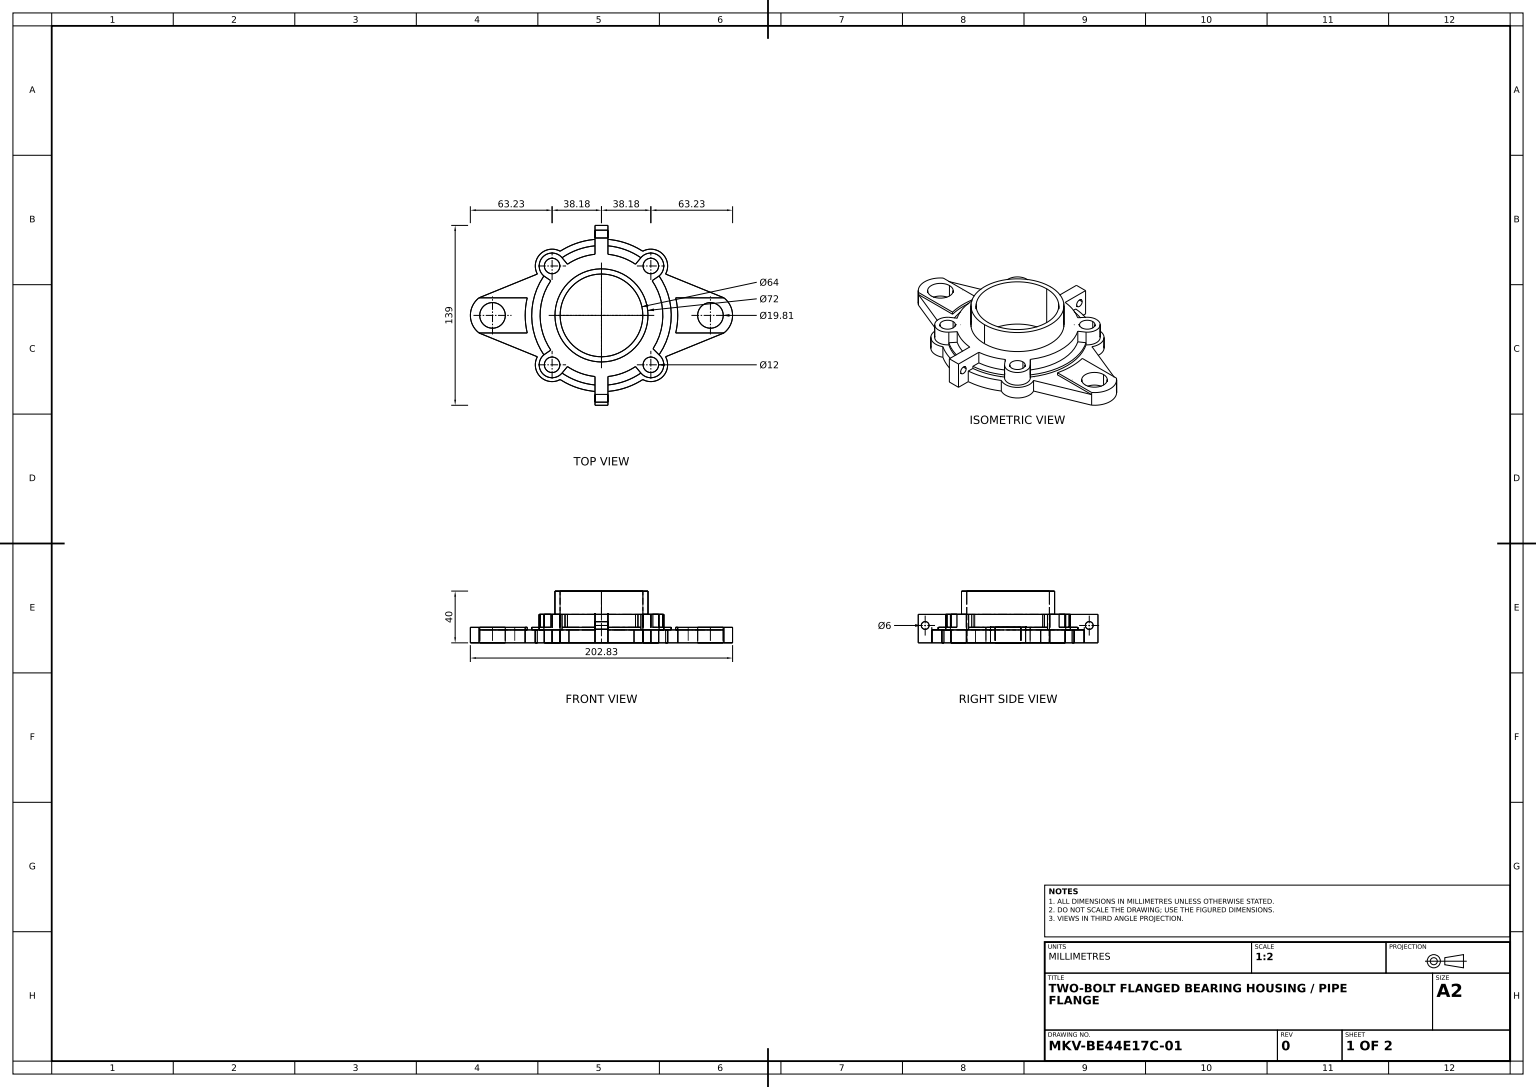
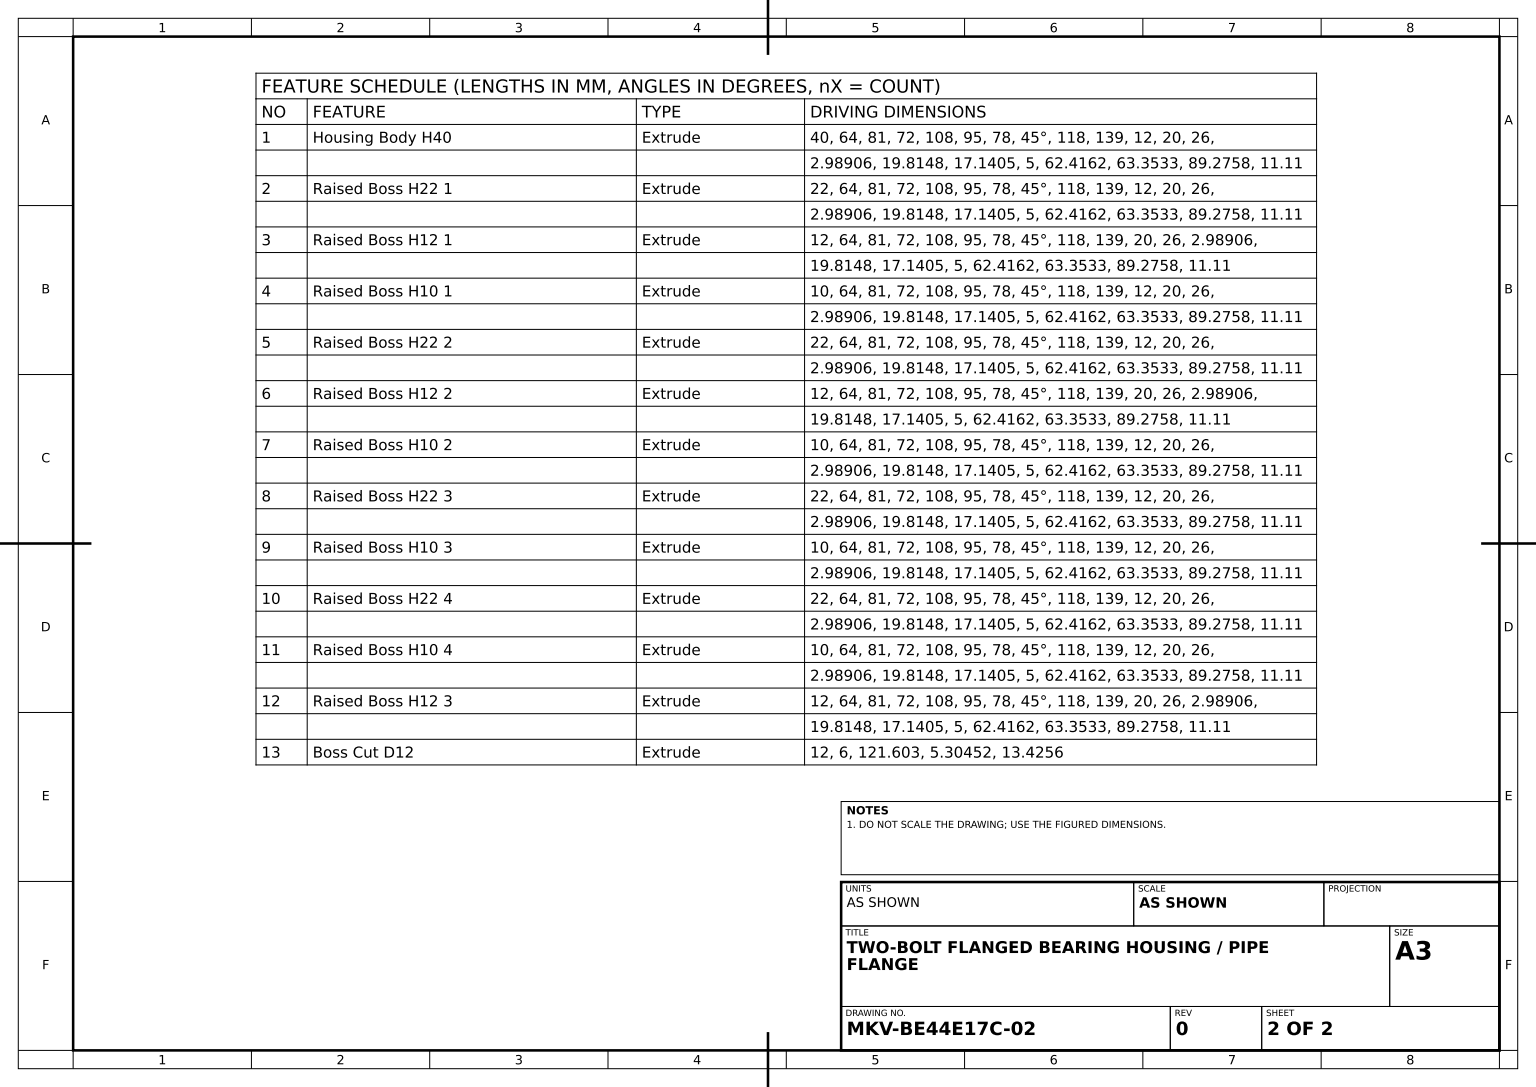
from build123d import *

# Parameters (mm, degrees)
HOUSING_LAYOUT_SKETCH_R   = 36
HOUSING_LAYOUT_SKETCH_R_2 = 32
HOUSING_BODY_H40_DEPTH    = 40
SKETCH1_7_R               = 36
RAISED_BOSS_H22_1_DEPTH   = 22
RAISED_BOSS_H12_1_DEPTH   = 12
RAISED_BOSS_H10_1_DEPTH   = 10
RAISED_BOSS_H22_2_DEPTH   = 22
RAISED_BOSS_H12_2_DEPTH   = 12
RAISED_BOSS_H10_2_DEPTH   = 10
RAISED_BOSS_H22_3_DEPTH   = 22
RAISED_BOSS_H10_3_DEPTH   = 10
RAISED_BOSS_H22_4_DEPTH   = 22
RAISED_BOSS_H10_4_DEPTH   = 10
SKETCH1_21_R              = 9.907401239
RAISED_BOSS_H12_3_DEPTH   = 12
BOSS_CUT_SKETCH_R         = 3
BOSS_CUT_D12_DEPTH        = 12


with BuildPart() as part:
    # Housing Layout Sketch → Housing Body H40 (new body)
    with BuildSketch(Plane(origin=(0, 0, 0), x_dir=(1, 0, 0), z_dir=(0, 1, 0))):
        with Locations(Location((0, 0, 0), (0, 0, 270))):
            Circle(HOUSING_LAYOUT_SKETCH_R)
        with Locations(Location((0, 0, 0), (0, 0, 270))):
            Circle(HOUSING_LAYOUT_SKETCH_R_2, mode=Mode.SUBTRACT)
    extrude(amount=HOUSING_BODY_H40_DEPTH)

    # Sketch1_7 → Raised Boss H22 1 (add)
    with BuildSketch(Plane(origin=(0, 0, 0), x_dir=(1, 0, 0), z_dir=(0, 1, 0))):
        with BuildLine():
            ThreePointArc((-5, 47.236109069), (-20.465112279, 42.865244423), (-33.587572106, 33.587572106))
            ThreePointArc((-33.587572106, 33.587572106), (-44.781324678, -15.839285339), (-5, -47.236109069))
            Line((-5, -47.236109069), (-5, -53.768020235))
            ThreePointArc((-5, -53.768020235), (0, -54), (5, -53.768020235))
            Line((5, -53.768020235), (5, -47.236109069))
            ThreePointArc((5, -47.236109069), (47.5, 0), (5, 47.236109069))
            Line((5, 47.236109069), (5, 53.768020235))
            ThreePointArc((5, 53.768020235), (0, 54), (-5, 53.768020235))
            Line((-5, 53.768020235), (-5, 47.236109069))
        make_face()
        with Locations(Location((0, 0, 0), (0, 0, 270))):
            Circle(SKETCH1_7_R, mode=Mode.SUBTRACT)
    extrude(amount=RAISED_BOSS_H22_1_DEPTH)

    # Sketch1_9 → Raised Boss H12 1 (add)
    with BuildSketch(Plane(origin=(0, 0, 0), x_dir=(1, 0, 0), z_dir=(0, 1, 0))):
        with BuildLine():
            ThreePointArc((-39.204853986, -26.818453049), (-47.5, 0), (-39.204853986, 26.818453049))
            Line((-39.204853986, 26.818453049), (-44.569728742, 30.488346624))
            ThreePointArc((-44.569728742, 30.488346624), (-54, 0), (-44.569728742, -30.488346624))
            Line((-44.569728742, -30.488346624), (-39.204853986, -26.818453049))
        make_face()
        with BuildLine():
            Line((44.569728742, 30.488346624), (39.204853986, 26.818453049))
            ThreePointArc((39.204853986, 26.818453049), (47.49606696, 0.611247373), (39.882031918, -25.8006498))
            Line((39.882031918, -25.8006498), (44.569728742, -30.488346624))
            ThreePointArc((44.569728742, -30.488346624), (54, 0), (44.569728742, 30.488346624))
        make_face()
    extrude(amount=RAISED_BOSS_H12_1_DEPTH)

    # Sketch1_10 → Raised Boss H10 1 (add)
    with BuildSketch(Plane(origin=(0, 0, 0), x_dir=(1, 0, 0), z_dir=(0, 1, 0))):
        with BuildLine():
            ThreePointArc((-44.569728742, -30.488346624), (-54, 0), (-44.569728742, 30.488346624))
            ThreePointArc((-44.569728742, 30.488346624), (-46.384787995, 32.461595157), (-47.610345509, 34.846161919))
            ThreePointArc((-47.610345509, 34.846161919), (-59, 0), (-47.610345509, -34.846161919))
            ThreePointArc((-47.610345509, -34.846161919), (-46.384787995, -32.461595157), (-44.569728742, -30.488346624))
        make_face()
        with BuildLine():
            ThreePointArc((47.610345509, -34.846161919), (59, 0), (47.610345509, 34.846161919))
            ThreePointArc((47.610345509, 34.846161919), (46.384787995, 32.461595157), (44.569728742, 30.488346624))
            ThreePointArc((44.569728742, 30.488346624), (54, 0), (44.569728742, -30.488346624))
            ThreePointArc((44.569728742, -30.488346624), (46.384787995, -32.461595157), (47.610345509, -34.846161919))
        make_face()
    extrude(amount=RAISED_BOSS_H10_1_DEPTH)

    # Sketch1_11 → Raised Boss H22 2 (add)
    with BuildSketch(Plane(origin=(0, 0, 0), x_dir=(1, 0, 0), z_dir=(0, 1, 0))):
        with BuildLine():
            ThreePointArc((5, -58.787753827), (0, -59), (-5, -58.787753827))
            Line((-5, -58.787753827), (-5, -69.463251536))
            Line((-5, -69.463251536), (5, -69.463251536))
            Line((5, -69.463251536), (5, -58.787753827))
        make_face()
        with BuildLine():
            Line((-5, 69.536748464), (-5, 58.787753827))
            ThreePointArc((-5, 58.787753827), (0, 59), (5, 58.787753827))
            Line((5, 58.787753827), (5, 69.536748464))
            Line((5, 69.536748464), (-5, 69.536748464))
        make_face()
        with BuildLine():
            Line((-5, 58.787753827), (-5, 53.768020235))
            ThreePointArc((-5, 53.768020235), (0, 54), (5, 53.768020235))
            Line((5, 53.768020235), (5, 58.787753827))
            ThreePointArc((5, 58.787753827), (0, 59), (-5, 58.787753827))
        make_face()
        with BuildLine():
            ThreePointArc((5, -53.768020235), (0, -54), (-5, -53.768020235))
            Line((-5, -53.768020235), (-5, -58.787753827))
            ThreePointArc((-5, -58.787753827), (0, -59), (5, -58.787753827))
            Line((5, -58.787753827), (5, -53.768020235))
        make_face()
    extrude(amount=RAISED_BOSS_H22_2_DEPTH)

    # Sketch1_14 → Raised Boss H12 2 (add)
    with BuildSketch(Plane(origin=(0, 0, 0), x_dir=(1, 0, 0), z_dir=(0, 1, 0))):
        with BuildLine():
            ThreePointArc((-5, -47.236109069), (-16.124065271, -44.679576085), (-26.31709261, -39.543149047))
            Line((-26.31709261, -39.543149047), (-30.488346624, -44.569728742))
            ThreePointArc((-30.488346624, -44.569728742), (-18.330516308, -50.793623339), (-5, -53.768020235))
            Line((-5, -53.768020235), (-5, -47.236109069))
        make_face()
        with BuildLine():
            Line((5, -47.236109069), (5, -53.768020235))
            ThreePointArc((5, -53.768020235), (18.330516308, -50.793623339), (30.488346624, -44.569728742))
            Line((30.488346624, -44.569728742), (26.31709261, -39.543149047))
            ThreePointArc((26.31709261, -39.543149047), (16.124065271, -44.679576085), (5, -47.236109069))
        make_face()
        with BuildLine():
            ThreePointArc((30.488346624, 44.569728742), (18.330516308, 50.793623339), (5, 53.768020235))
            Line((5, 53.768020235), (5, 47.236109069))
            ThreePointArc((5, 47.236109069), (16.124065271, 44.679576085), (26.31709261, 39.543149047))
            Line((26.31709261, 39.543149047), (30.488346624, 44.569728742))
        make_face()
        with BuildLine():
            Line((-30.488346624, 44.569728742), (-26.31709261, 39.543149047))
            ThreePointArc((-26.31709261, 39.543149047), (-16.124065271, 44.679576085), (-5, 47.236109069))
            Line((-5, 47.236109069), (-5, 53.768020235))
            ThreePointArc((-5, 53.768020235), (-18.330516308, 50.793623339), (-30.488346624, 44.569728742))
        make_face()
    extrude(amount=RAISED_BOSS_H12_2_DEPTH)

    # Sketch1_15 → Raised Boss H10 2 (add)
    with BuildSketch(Plane(origin=(0, 0, 0), x_dir=(1, 0, 0), z_dir=(0, 1, 0))):
        with BuildLine():
            ThreePointArc((-5, -53.768020235), (-18.330516308, -50.793623339), (-30.488346624, -44.569728742))
            ThreePointArc((-30.488346624, -44.569728742), (-32.461595157, -46.384787995), (-34.846161919, -47.610345509))
            ThreePointArc((-34.846161919, -47.610345509), (-33.416487996, -48.624462259), (-31.957320012, -49.595662085))
            ThreePointArc((-31.957320012, -49.595662085), (-19.041652062, -55.842774705), (-5, -58.787753827))
            Line((-5, -58.787753827), (-5, -53.768020235))
        make_face()
        with BuildLine():
            ThreePointArc((30.488346624, -44.569728742), (18.330516308, -50.793623339), (5, -53.768020235))
            Line((5, -53.768020235), (5, -58.787753827))
            ThreePointArc((5, -58.787753827), (19.041652062, -55.842774705), (31.957320012, -49.595662085))
            ThreePointArc((31.957320012, -49.595662085), (33.416487996, -48.624462259), (34.846161919, -47.610345509))
            ThreePointArc((34.846161919, -47.610345509), (32.461595157, -46.384787995), (30.488346624, -44.569728742))
        make_face()
        with BuildLine():
            ThreePointArc((-34.846161919, 47.610345509), (-32.461595157, 46.384787995), (-30.488346624, 44.569728742))
            ThreePointArc((-30.488346624, 44.569728742), (-18.330516308, 50.793623339), (-5, 53.768020235))
            Line((-5, 53.768020235), (-5, 58.787753827))
            ThreePointArc((-5, 58.787753827), (-19.041652062, 55.842774705), (-31.957320012, 49.595662085))
            ThreePointArc((-31.957320012, 49.595662085), (-33.416487996, 48.624462259), (-34.846161919, 47.610345509))
        make_face()
        with BuildLine():
            Line((5, 58.787753827), (5, 53.768020235))
            ThreePointArc((5, 53.768020235), (18.330516308, 50.793623339), (30.488346624, 44.569728742))
            ThreePointArc((30.488346624, 44.569728742), (32.461595157, 46.384787995), (34.846161919, 47.610345509))
            ThreePointArc((34.846161919, 47.610345509), (33.416487996, 48.624462259), (31.957320012, 49.595662085))
            ThreePointArc((31.957320012, 49.595662085), (19.041652062, 55.842774705), (5, 58.787753827))
        make_face()
    extrude(amount=RAISED_BOSS_H10_2_DEPTH)

    # Sketch1_16 → Raised Boss H22 3 (add)
    with BuildSketch(Plane(origin=(0, 0, 0), x_dir=(1, 0, 0), z_dir=(0, 1, 0))):
        with BuildLine():
            ThreePointArc((-26.31709261, -39.543149047), (-33.373055651, -33.800727159), (-39.204853986, -26.818453049))
            Line((-39.204853986, -26.818453049), (-44.569728742, -30.488346624))
            ThreePointArc((-44.569728742, -30.488346624), (-43.406876338, -32.122314465), (-42.184152266, -33.711975581))
            ThreePointArc((-42.184152266, -33.711975581), (-35.734512879, -32.706434877), (-32.183766184, -38.183766184))
            ThreePointArc((-32.183766184, -38.183766184), (-32.578824453, -40.324940673), (-33.711975581, -42.184152266))
            ThreePointArc((-33.711975581, -42.184152266), (-32.122314465, -43.406876338), (-30.488346624, -44.569728742))
            Line((-30.488346624, -44.569728742), (-26.31709261, -39.543149047))
        make_face()
        with BuildLine():
            ThreePointArc((-39.204853986, 26.818453049), (-36.553242911, 30.333322151), (-33.587572106, 33.587572106))
            Line((-33.587572106, 33.587572106), (-33.941125497, 33.941125497))
            ThreePointArc((-33.941125497, 33.941125497), (-38.01703513, 32.186083235), (-42.184152266, 33.711975581))
            ThreePointArc((-42.184152266, 33.711975581), (-43.406876338, 32.122314465), (-44.569728742, 30.488346624))
            Line((-44.569728742, 30.488346624), (-39.204853986, 26.818453049))
        make_face()
        with BuildLine():
            Line((-33.941125497, 33.941125497), (-33.587572106, 33.587572106))
            ThreePointArc((-33.587572106, 33.587572106), (-30.099990662, 36.745619632), (-26.31709261, 39.543149047))
            Line((-26.31709261, 39.543149047), (-30.488346624, 44.569728742))
            ThreePointArc((-30.488346624, 44.569728742), (-32.122314465, 43.406876338), (-33.711975581, 42.184152266))
            ThreePointArc((-33.711975581, 42.184152266), (-32.578824453, 40.324940673), (-32.183766184, 38.183766184))
            ThreePointArc((-32.183766184, 38.183766184), (-32.640488989, 35.88766559), (-33.941125497, 33.941125497))
        make_face()
        with BuildLine():
            ThreePointArc((33.711975581, 42.184152266), (32.122314465, 43.406876338), (30.488346624, 44.569728742))
            Line((30.488346624, 44.569728742), (26.31709261, 39.543149047))
            ThreePointArc((26.31709261, 39.543149047), (33.373055651, 33.800727159), (39.204853986, 26.818453049))
            Line((39.204853986, 26.818453049), (44.569728742, 30.488346624))
            ThreePointArc((44.569728742, 30.488346624), (43.406876338, 32.122314465), (42.184152266, 33.711975581))
            ThreePointArc((42.184152266, 33.711975581), (33.941125497, 33.941125497), (33.711975581, 42.184152266))
        make_face()
    extrude(amount=RAISED_BOSS_H22_3_DEPTH)

    # Sketch1_18 → Raised Boss H10 3 (add)
    with BuildSketch(Plane(origin=(0, 0, 0), x_dir=(1, 0, 0), z_dir=(0, 1, 0))):
        with BuildLine():
            ThreePointArc((49.595662085, 31.957320012), (47.376154339, 47.376154339), (31.957320012, 49.595662085))
            ThreePointArc((31.957320012, 49.595662085), (33.416487996, 48.624462259), (34.846161919, 47.610345509))
            ThreePointArc((34.846161919, 47.610345509), (45.254833996, 45.254833996), (47.610345509, 34.846161919))
            ThreePointArc((47.610345509, 34.846161919), (48.624462259, 33.416487996), (49.595662085, 31.957320012))
        make_face()
        with BuildLine():
            ThreePointArc((-47.610345509, 34.846161919), (-45.254833996, 45.254833996), (-34.846161919, 47.610345509))
            ThreePointArc((-34.846161919, 47.610345509), (-33.416487996, 48.624462259), (-31.957320012, 49.595662085))
            ThreePointArc((-31.957320012, 49.595662085), (-47.376154339, 47.376154339), (-49.595662085, 31.957320012))
            ThreePointArc((-49.595662085, 31.957320012), (-48.624462259, 33.416487996), (-47.610345509, 34.846161919))
        make_face()
        with BuildLine():
            ThreePointArc((-34.846161919, -47.610345509), (-45.254833996, -45.254833996), (-47.610345509, -34.846161919))
            ThreePointArc((-47.610345509, -34.846161919), (-48.624462259, -33.416487996), (-49.595662085, -31.957320012))
            ThreePointArc((-49.595662085, -31.957320012), (-47.376154339, -47.376154339), (-31.957320012, -49.595662085))
            ThreePointArc((-31.957320012, -49.595662085), (-33.416487996, -48.624462259), (-34.846161919, -47.610345509))
        make_face()
        with BuildLine():
            ThreePointArc((34.846161919, -47.610345509), (33.416487996, -48.624462259), (31.957320012, -49.595662085))
            ThreePointArc((31.957320012, -49.595662085), (47.376154339, -47.376154339), (49.595662085, -31.957320012))
            ThreePointArc((49.595662085, -31.957320012), (48.624462259, -33.416487996), (47.610345509, -34.846161919))
            ThreePointArc((47.610345509, -34.846161919), (45.254833996, -45.254833996), (34.846161919, -47.610345509))
        make_face()
    extrude(amount=RAISED_BOSS_H10_3_DEPTH)

    # Sketch1_19 → Raised Boss H22 4 (add)
    with BuildSketch(Plane(origin=(0, 0, 0), x_dir=(1, 0, 0), z_dir=(0, 1, 0))):
        with BuildLine():
            ThreePointArc((39.196959086, -44.097600824), (37.063199887, -45.90554666), (34.846161919, -47.610345509))
            ThreePointArc((34.846161919, -47.610345509), (45.254833996, -45.254833996), (47.610345509, -34.846161919))
            ThreePointArc((47.610345509, -34.846161919), (45.90554666, -37.063199887), (44.097600824, -39.196959086))
            ThreePointArc((44.097600824, -39.196959086), (42.426406871, -42.426406871), (39.196959086, -44.097600824))
        make_face()
        with BuildLine():
            Line((26.31709261, -39.543149047), (30.488346624, -44.569728742))
            ThreePointArc((30.488346624, -44.569728742), (32.122314465, -43.406876338), (33.711975581, -42.184152266))
            ThreePointArc((33.711975581, -42.184152266), (33.941125497, -33.941125497), (42.184152266, -33.711975581))
            ThreePointArc((42.184152266, -33.711975581), (43.406876338, -32.122314465), (44.569728742, -30.488346624))
            Line((44.569728742, -30.488346624), (39.882031918, -25.8006498))
            ThreePointArc((39.882031918, -25.8006498), (33.805252454, -33.368471744), (26.31709261, -39.543149047))
        make_face()
        with BuildLine():
            ThreePointArc((33.711975581, -42.184152266), (32.122314465, -43.406876338), (30.488346624, -44.569728742))
            ThreePointArc((30.488346624, -44.569728742), (32.461595157, -46.384787995), (34.846161919, -47.610345509))
            ThreePointArc((34.846161919, -47.610345509), (37.063199887, -45.90554666), (39.196959086, -44.097600824))
            ThreePointArc((39.196959086, -44.097600824), (36.207457539, -43.848940863), (33.711975581, -42.184152266))
        make_face()
        with BuildLine():
            ThreePointArc((47.610345509, -34.846161919), (46.384787995, -32.461595157), (44.569728742, -30.488346624))
            ThreePointArc((44.569728742, -30.488346624), (43.406876338, -32.122314465), (42.184152266, -33.711975581))
            ThreePointArc((42.184152266, -33.711975581), (43.661097491, -35.734512879), (44.183766184, -38.183766184))
            ThreePointArc((44.183766184, -38.183766184), (44.162186035, -38.692191283), (44.097600824, -39.196959086))
            ThreePointArc((44.097600824, -39.196959086), (45.90554666, -37.063199887), (47.610345509, -34.846161919))
        make_face()
        with BuildLine():
            ThreePointArc((33.711975581, -42.184152266), (32.122314465, -43.406876338), (30.488346624, -44.569728742))
            ThreePointArc((30.488346624, -44.569728742), (32.461595157, -46.384787995), (34.846161919, -47.610345509))
            ThreePointArc((34.846161919, -47.610345509), (37.063199887, -45.90554666), (39.196959086, -44.097600824))
            ThreePointArc((39.196959086, -44.097600824), (36.207457539, -43.848940863), (33.711975581, -42.184152266))
        make_face()
        with BuildLine():
            ThreePointArc((47.610345509, -34.846161919), (46.384787995, -32.461595157), (44.569728742, -30.488346624))
            ThreePointArc((44.569728742, -30.488346624), (43.406876338, -32.122314465), (42.184152266, -33.711975581))
            ThreePointArc((42.184152266, -33.711975581), (43.661097491, -35.734512879), (44.183766184, -38.183766184))
            ThreePointArc((44.183766184, -38.183766184), (44.162186035, -38.692191283), (44.097600824, -39.196959086))
            ThreePointArc((44.097600824, -39.196959086), (45.90554666, -37.063199887), (47.610345509, -34.846161919))
        make_face()
        with BuildLine():
            ThreePointArc((-44.097600824, -39.196959086), (-45.90554666, -37.063199887), (-47.610345509, -34.846161919))
            ThreePointArc((-47.610345509, -34.846161919), (-45.254833996, -45.254833996), (-34.846161919, -47.610345509))
            ThreePointArc((-34.846161919, -47.610345509), (-37.063199887, -45.90554666), (-39.196959086, -44.097600824))
            ThreePointArc((-39.196959086, -44.097600824), (-42.426406871, -42.426406871), (-44.097600824, -39.196959086))
        make_face()
        with BuildLine():
            ThreePointArc((-42.184152266, -33.711975581), (-43.406876338, -32.122314465), (-44.569728742, -30.488346624))
            ThreePointArc((-44.569728742, -30.488346624), (-46.384787995, -32.461595157), (-47.610345509, -34.846161919))
            ThreePointArc((-47.610345509, -34.846161919), (-45.90554666, -37.063199887), (-44.097600824, -39.196959086))
            ThreePointArc((-44.097600824, -39.196959086), (-43.848940863, -36.207457539), (-42.184152266, -33.711975581))
        make_face()
        with BuildLine():
            ThreePointArc((-34.846161919, -47.610345509), (-32.461595157, -46.384787995), (-30.488346624, -44.569728742))
            ThreePointArc((-30.488346624, -44.569728742), (-32.122314465, -43.406876338), (-33.711975581, -42.184152266))
            ThreePointArc((-33.711975581, -42.184152266), (-36.207457539, -43.848940863), (-39.196959086, -44.097600824))
            ThreePointArc((-39.196959086, -44.097600824), (-37.063199887, -45.90554666), (-34.846161919, -47.610345509))
        make_face()
        with BuildLine():
            ThreePointArc((-42.184152266, -33.711975581), (-43.406876338, -32.122314465), (-44.569728742, -30.488346624))
            ThreePointArc((-44.569728742, -30.488346624), (-46.384787995, -32.461595157), (-47.610345509, -34.846161919))
            ThreePointArc((-47.610345509, -34.846161919), (-45.90554666, -37.063199887), (-44.097600824, -39.196959086))
            ThreePointArc((-44.097600824, -39.196959086), (-43.848940863, -36.207457539), (-42.184152266, -33.711975581))
        make_face()
        with BuildLine():
            ThreePointArc((-34.846161919, -47.610345509), (-32.461595157, -46.384787995), (-30.488346624, -44.569728742))
            ThreePointArc((-30.488346624, -44.569728742), (-32.122314465, -43.406876338), (-33.711975581, -42.184152266))
            ThreePointArc((-33.711975581, -42.184152266), (-36.207457539, -43.848940863), (-39.196959086, -44.097600824))
            ThreePointArc((-39.196959086, -44.097600824), (-37.063199887, -45.90554666), (-34.846161919, -47.610345509))
        make_face()
        with BuildLine():
            ThreePointArc((34.846161919, 47.610345509), (32.461595157, 46.384787995), (30.488346624, 44.569728742))
            ThreePointArc((30.488346624, 44.569728742), (32.122314465, 43.406876338), (33.711975581, 42.184152266))
            ThreePointArc((33.711975581, 42.184152266), (36.207457539, 43.848940863), (39.196959086, 44.097600824))
            ThreePointArc((39.196959086, 44.097600824), (37.063199887, 45.90554666), (34.846161919, 47.610345509))
        make_face()
        with BuildLine():
            ThreePointArc((44.183766184, 38.183766184), (43.661097491, 35.734512879), (42.184152266, 33.711975581))
            ThreePointArc((42.184152266, 33.711975581), (43.406876338, 32.122314465), (44.569728742, 30.488346624))
            ThreePointArc((44.569728742, 30.488346624), (46.384787995, 32.461595157), (47.610345509, 34.846161919))
            ThreePointArc((47.610345509, 34.846161919), (45.90554666, 37.063199887), (44.097600824, 39.196959086))
            ThreePointArc((44.097600824, 39.196959086), (44.162186035, 38.692191283), (44.183766184, 38.183766184))
        make_face()
        with BuildLine():
            ThreePointArc((34.846161919, 47.610345509), (32.461595157, 46.384787995), (30.488346624, 44.569728742))
            ThreePointArc((30.488346624, 44.569728742), (32.122314465, 43.406876338), (33.711975581, 42.184152266))
            ThreePointArc((33.711975581, 42.184152266), (36.207457539, 43.848940863), (39.196959086, 44.097600824))
            ThreePointArc((39.196959086, 44.097600824), (37.063199887, 45.90554666), (34.846161919, 47.610345509))
        make_face()
        with BuildLine():
            ThreePointArc((44.183766184, 38.183766184), (43.661097491, 35.734512879), (42.184152266, 33.711975581))
            ThreePointArc((42.184152266, 33.711975581), (43.406876338, 32.122314465), (44.569728742, 30.488346624))
            ThreePointArc((44.569728742, 30.488346624), (46.384787995, 32.461595157), (47.610345509, 34.846161919))
            ThreePointArc((47.610345509, 34.846161919), (45.90554666, 37.063199887), (44.097600824, 39.196959086))
            ThreePointArc((44.097600824, 39.196959086), (44.162186035, 38.692191283), (44.183766184, 38.183766184))
        make_face()
        with BuildLine():
            ThreePointArc((47.610345509, 34.846161919), (45.254833996, 45.254833996), (34.846161919, 47.610345509))
            ThreePointArc((34.846161919, 47.610345509), (37.063199887, 45.90554666), (39.196959086, 44.097600824))
            ThreePointArc((39.196959086, 44.097600824), (42.426406871, 42.426406871), (44.097600824, 39.196959086))
            ThreePointArc((44.097600824, 39.196959086), (45.90554666, 37.063199887), (47.610345509, 34.846161919))
        make_face()
        with BuildLine():
            ThreePointArc((-47.610345509, 34.846161919), (-45.90554666, 37.063199887), (-44.097600824, 39.196959086))
            ThreePointArc((-44.097600824, 39.196959086), (-42.426406871, 42.426406871), (-39.196959086, 44.097600824))
            ThreePointArc((-39.196959086, 44.097600824), (-37.063199887, 45.90554666), (-34.846161919, 47.610345509))
            ThreePointArc((-34.846161919, 47.610345509), (-45.254833996, 45.254833996), (-47.610345509, 34.846161919))
        make_face()
        with BuildLine():
            ThreePointArc((-44.569728742, 30.488346624), (-43.406876338, 32.122314465), (-42.184152266, 33.711975581))
            ThreePointArc((-42.184152266, 33.711975581), (-43.848940863, 36.207457539), (-44.097600824, 39.196959086))
            ThreePointArc((-44.097600824, 39.196959086), (-45.90554666, 37.063199887), (-47.610345509, 34.846161919))
            ThreePointArc((-47.610345509, 34.846161919), (-46.384787995, 32.461595157), (-44.569728742, 30.488346624))
        make_face()
        with BuildLine():
            ThreePointArc((-33.711975581, 42.184152266), (-32.122314465, 43.406876338), (-30.488346624, 44.569728742))
            ThreePointArc((-30.488346624, 44.569728742), (-32.461595157, 46.384787995), (-34.846161919, 47.610345509))
            ThreePointArc((-34.846161919, 47.610345509), (-37.063199887, 45.90554666), (-39.196959086, 44.097600824))
            ThreePointArc((-39.196959086, 44.097600824), (-36.207457539, 43.848940863), (-33.711975581, 42.184152266))
        make_face()
        with BuildLine():
            ThreePointArc((-44.569728742, 30.488346624), (-43.406876338, 32.122314465), (-42.184152266, 33.711975581))
            ThreePointArc((-42.184152266, 33.711975581), (-43.848940863, 36.207457539), (-44.097600824, 39.196959086))
            ThreePointArc((-44.097600824, 39.196959086), (-45.90554666, 37.063199887), (-47.610345509, 34.846161919))
            ThreePointArc((-47.610345509, 34.846161919), (-46.384787995, 32.461595157), (-44.569728742, 30.488346624))
        make_face()
        with BuildLine():
            ThreePointArc((-33.711975581, 42.184152266), (-32.122314465, 43.406876338), (-30.488346624, 44.569728742))
            ThreePointArc((-30.488346624, 44.569728742), (-32.461595157, 46.384787995), (-34.846161919, 47.610345509))
            ThreePointArc((-34.846161919, 47.610345509), (-37.063199887, 45.90554666), (-39.196959086, 44.097600824))
            ThreePointArc((-39.196959086, 44.097600824), (-36.207457539, 43.848940863), (-33.711975581, 42.184152266))
        make_face()
    extrude(amount=RAISED_BOSS_H22_4_DEPTH)

    # Sketch1_20 → Raised Boss H10 4 (add)
    with BuildSketch(Plane(origin=(0, 0, 0), x_dir=(1, 0, 0), z_dir=(0, 1, 0))):
        with BuildLine():
            Line((49.595662085, -31.957320012), (94.736257942, -13.578493986))
            Line((94.736257942, -13.578493986), (57.416239001, -13.578493986))
            ThreePointArc((57.416239001, -13.578493986), (54.289336477, -23.101254185), (49.595662085, -31.957320012))
        make_face()
        with BuildLine():
            Line((94.736257942, 13.578493986), (49.595662085, 31.957320012))
            ThreePointArc((49.595662085, 31.957320012), (54.289336477, 23.101254185), (57.416239001, 13.578493986))
            Line((57.416239001, 13.578493986), (94.736257942, 13.578493986))
        make_face()
        with BuildLine():
            Line((-94.736257942, -13.578493986), (-49.595662085, -31.957320012))
            ThreePointArc((-49.595662085, -31.957320012), (-54.289336477, -23.101254185), (-57.416239001, -13.578493986))
            Line((-57.416239001, -13.578493986), (-94.736257942, -13.578493986))
        make_face()
        with BuildLine():
            ThreePointArc((-57.416239001, 13.578493986), (-54.289336477, 23.101254185), (-49.595662085, 31.957320012))
            Line((-49.595662085, 31.957320012), (-94.736257942, 13.578493986))
            Line((-94.736257942, 13.578493986), (-57.416239001, 13.578493986))
        make_face()
    extrude(amount=RAISED_BOSS_H10_4_DEPTH)

    # Sketch1_21 → Raised Boss H12 3 (add)
    # profile 1 of 2: a face of its own
    with BuildSketch(Plane(origin=(0, 0, 0), x_dir=(1, 0, 0), z_dir=(0, 1, 0))):
        with BuildLine():
            ThreePointArc((94.736257942, -13.578493986), (101.416291697, 0), (94.736257942, 13.578493986))
            Line((94.736257942, 13.578493986), (57.416239001, 13.578493986))
            ThreePointArc((57.416239001, 13.578493986), (58.602722211, 6.835272449), (59, 0))
            ThreePointArc((59, 0), (58.602722211, -6.835272449), (57.416239001, -13.578493986))
            Line((57.416239001, -13.578493986), (94.736257942, -13.578493986))
        make_face()
        with Locations(Location((84.275783259, 0, 0), (0, 0, 270))):
            Circle(SKETCH1_21_R, mode=Mode.SUBTRACT)
    # profile 2 of 2: a face of its own
    with BuildSketch(Plane(origin=(0, 0, 0), x_dir=(1, 0, 0), z_dir=(0, 1, 0))):
        with BuildLine():
            Line((-57.416239001, 13.578493986), (-94.736257942, 13.578493986))
            ThreePointArc((-94.736257942, 13.578493986), (-101.416291697, 0), (-94.736257942, -13.578493986))
            Line((-94.736257942, -13.578493986), (-57.416239001, -13.578493986))
            ThreePointArc((-57.416239001, -13.578493986), (-59, 0), (-57.416239001, 13.578493986))
        make_face()
        with Locations(Location((-84.275783259, 0, 0), (0, 0, 270))):
            Circle(SKETCH1_21_R, mode=Mode.SUBTRACT)
    extrude(amount=RAISED_BOSS_H12_3_DEPTH)

    # Boss Cut Sketch → Boss Cut D12 (cut)
    with BuildSketch(Plane(origin=(5, 0, 0), x_dir=(0, 0, -1), z_dir=(1, 0, 0))):
        with Locations((-64.092276099, 13.425612095)):
            Circle(BOSS_CUT_SKETCH_R)
        with Locations((62.815285265, 13.425612095)):
            Circle(BOSS_CUT_SKETCH_R)
    extrude(amount=-BOSS_CUT_D12_DEPTH, mode=Mode.SUBTRACT)


solid = part.part
